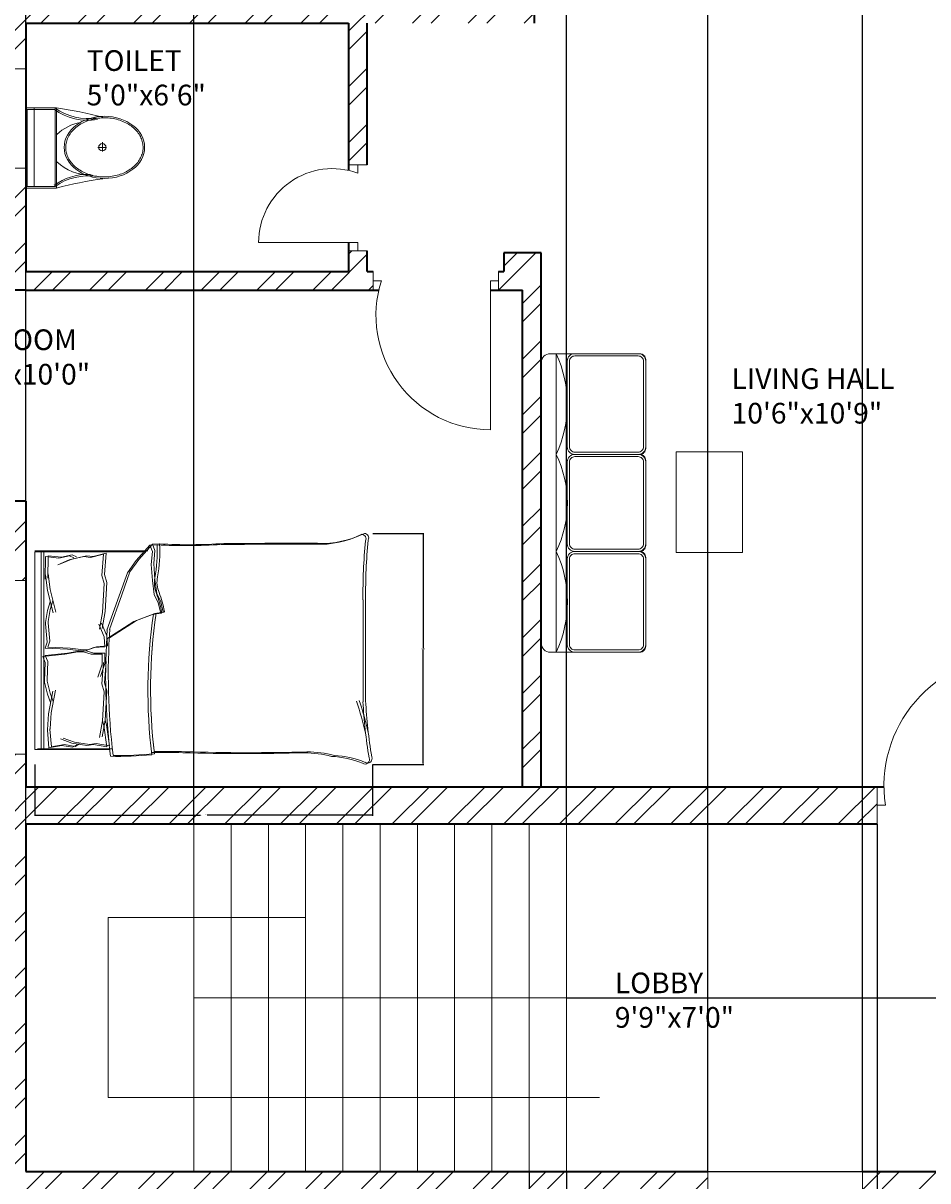
# Model space of a CAD drawing. Units: inches. Extents: x 1513 to 2170, y 1240 to 2288.
# Tile 8 of 10: x 1623 to 1842, y 1801 to 2081. Entities that reach past the tile are written whole.
import ezdxf

# ---------------------------------------------------------------- set-up
doc = ezdxf.new("R2010")
doc.units = ezdxf.units.IN
for name, color, linetype, lineweight in [('A-ANNO-DIMS', 2, 'Continuous', 18), ('A-AREA-IDEN', 7, 'Continuous', 18), ('A-DOOR', 3, 'Continuous', 18), ('A-FLOR-FIXT', 9, 'Continuous', 18), ('A-FLOR-STRS', 7, 'Continuous', 18), ('A-FURN', 8, 'Continuous', 18), ('A-GLAZ', 4, 'Continuous', 18), ('A-WALL', 7, 'Continuous', 35), ('A-WALL-PATT', 252, 'Continuous', 13)]:
    doc.layers.add(name, color=color, linetype=linetype, lineweight=lineweight)
doc.styles.get("Standard").update_dxf_attribs({"font": 'arial.ttf'})
doc.dimstyles.get("Standard").update_dxf_attribs({"dimtxt": 0.18, "dimasz": 0.18, "dimexe": 0.18, "dimexo": 0.0625, "dimgap": 0.09, "dimtad": 0, "dimtih": 1, "dimtoh": 1, "dimdec": 4, "dimzin": 0, "dimdsep": 46, "dimtxsty": 'Standard', "dimcen": 0.09, "dimadec": 0, "dimazin": 0, "dimtfac": 1, "dimtdec": 4, "dimtofl": 0, "dimtmove": 0, "dimatfit": 3, "dimfxl": 1, "dimtolj": 1, "dimtzin": 0, "dimarcsym": 0})

# ---------------------------------------------------------------- blocks, each defined once
blk = doc.blocks.new('A$C31115884')
for p, q in [((283.1, 497.7), (223.4, 497.7)), ((257.5, 466.4), (257.5, 523.2)), ((0, 200), (0, 0)), ((520, 200), (0, 200)), ((10, 190), (10, 10)), ((510, 190), (10, 190)), ((510, 10), (510, 190)), ((520, 0), (520, 200)), ((510, 54.5), (0, 54.5)), ((10, 10), (510, 10)), ((0, 0), (520, 0))]:
    blk.add_line(p, q)
blk.add_circle((255.6, 496.4), 23.6)
for centre, radius, start, end in [((2777.7, -204.6), 2807, 165.4549, 171.71327), ((-294.5, 403.3), 364.7, 324.20913, 9.34987), ((-294.5, 403.3), 374.7, 324.20913, 9.34987), ((805.8, 403.3), 364.7, 170.65013, 215.79087), ((3237, 905), 2807, 188.28673, 194.5451), ((139.5, 406.2), 293.5, 315.84364, 2.65635), ((805.8, 403.3), 374.7, 179.20365, 215.79087), ((383.6, 406.2), 293.5, 190.27735, 224.15636)]:
    blk.add_arc(centre, radius, start, end)
blk.add_ellipse((256.2, 509.9), major_axis=(0, -260.7), ratio=0.772727)
blk.add_open_spline([(256.2, 259.2), (263.1, 259.2), (270, 259.7), (287.8, 262.3), (298.7, 265.1), (319.9, 273.1), (330.2, 278.4), (350.1, 291.1), (359.7, 298.7), (377.7, 315.9), (386.2, 325.5), (401.7, 346.6), (408.8, 358.1), (421.3, 382.5), (426.8, 395.5), (435.9, 422.4), (439.5, 436.4), (444.8, 465.1), (446.5, 479.7), (447.9, 509.2), (447.6, 524), (445, 553.3), (442.7, 567.8), (436.3, 596), (432.1, 609.7), (421.9, 636), (416, 648.6), (402.5, 672.1), (395, 683), (378.6, 703), (369.8, 712.1), (351.1, 728), (341.3, 734.8), (320.9, 746.2), (310.4, 750.7), (288.9, 757.3), (278, 759.4), (256, 761), (245, 760.6), (223.1, 757.2), (212.3, 754.3), (191.1, 746.1), (180.8, 740.7), (160.9, 727.8), (151.4, 720.1), (133.5, 702.7), (125.1, 693), (109.6, 671.7), (102.6, 660.2), (90.2, 635.7), (84.9, 622.7), (76, 595.6), (72.4, 581.6), (67.2, 552.9), (65.6, 538.2), (64.4, 508.8), (64.8, 494), (67.5, 464.7), (69.9, 450.2), (76.6, 422), (80.8, 408.3), (91.1, 382.2), (97.2, 369.7), (110.8, 346.3), (118.4, 335.4), (134.8, 315.6), (143.7, 306.7), (162.4, 290.9), (172.3, 284.2), (192.8, 273), (203.3, 268.6), (224.8, 262.2), (235.8, 260.2), (249.9, 259.3), (253, 259.2), (256.2, 259.2)], degree=3, knots=[0, 0, 0, 0, 0.110105, 0.110105, 0.285049, 0.285049, 0.459994, 0.459994, 0.634938, 0.634938, 0.809882, 0.809882, 0.984827, 0.984827, 1.159771, 1.159771, 1.334715, 1.334715, 1.50966, 1.50966, 1.684604, 1.684604, 1.859549, 1.859549, 2.034493, 2.034493, 2.209437, 2.209437, 2.384382, 2.384382, 2.559326, 2.559326, 2.73427, 2.73427, 2.909215, 2.909215, 3.084159, 3.084159, 3.259103, 3.259103, 3.434048, 3.434048, 3.608992, 3.608992, 3.783936, 3.783936, 3.958881, 3.958881, 4.133825, 4.133825, 4.30877, 4.30877, 4.483714, 4.483714, 4.658658, 4.658658, 4.833603, 4.833603, 5.008547, 5.008547, 5.183491, 5.183491, 5.358436, 5.358436, 5.53338, 5.53338, 5.708324, 5.708324, 5.883269, 5.883269, 6.058213, 6.058213, 6.233158, 6.233158, 6.283185, 6.283185, 6.283185, 6.283185])
blk = doc.blocks.new('BED-DOUBLE')
for p, q in [((30.13, 53.18), (28.38, 53.1, 3.87)), ((30.13, 53.18), (28.38, 53.1, 3.87)), ((0, 51.27), (26.61, 51.27)), ((0, 51.27), (26.61, 51.27)), ((0.64, 51.49), (27.25, 51.49)), ((0.64, 51.49), (27.25, 51.49)), ((1.53, 3.48), (1.53, 51.27)), ((1.53, 3.48), (1.53, 51.27)), ((2.17, 3.7), (2.17, 51.49)), ((2.17, 3.7), (2.17, 51.49)), ((6.4, 49.96), (8.97, 50.56)), ((6.4, 49.96), (8.97, 50.56)), ((8.97, 50.56), (10.02, 50.04)), ((8.97, 50.56), (10.02, 50.04)), ((16.57, 50.7), (13.43, 49.92)), ((16.57, 50.7), (13.43, 49.92)), ((17.21, 50.93), (14.07, 50.15)), ((17.21, 50.93), (14.07, 50.15)), ((16.17, 45.57), (16.57, 50.7)), ((16.17, 45.57), (16.57, 50.7)), ((16.8, 45.8), (17.21, 50.93)), ((16.8, 45.8), (17.21, 50.93)), ((27.74, 52.87), (24.49, 49.16)), ((27.74, 52.87), (24.49, 49.16)), ((28.38, 53.1), (25.13, 49.39)), ((28.38, 53.1), (25.13, 49.39)), ((29.49, 52.95), (27.74, 52.87, 3.87)), ((29.49, 52.95), (27.74, 52.87, 3.87)), ((28.36, 51.33), (27.74, 52.87)), ((28.36, 51.33), (27.74, 52.87)), ((28.05, 48.23), (28.36, 51.33)), ((28.05, 48.23), (28.36, 51.33)), ((29, 51.56), (28.38, 53.1)), ((29, 51.56), (28.38, 53.1)), ((28.69, 48.46), (29, 51.56)), ((28.69, 48.46), (29, 51.56)), ((2.55, 50.11), (2.46, 44.71)), ((2.55, 50.11), (2.46, 44.71)), ((2.55, 50.11), (5.76, 49.73)), ((2.55, 50.11), (5.76, 49.73)), ((3.19, 50.34), (3.1, 44.94)), ((3.19, 50.34), (3.1, 44.94)), ((3.19, 50.34), (6.4, 49.96)), ((3.19, 50.34), (6.4, 49.96)), ((8.25, 49.31), (5.57, 48.13)), ((8.25, 49.31), (5.57, 48.13)), ((5.76, 49.73), (8.33, 50.33)), ((5.76, 49.73), (8.33, 50.33)), ((8.89, 49.54), (6.21, 48.36)), ((8.89, 49.54), (6.21, 48.36)), ((11.83, 50.11), (8.25, 49.31)), ((11.83, 50.11), (8.25, 49.31)), ((8.33, 50.33), (9.38, 49.82)), ((8.33, 50.33), (9.38, 49.82)), ((12.46, 50.34), (8.89, 49.54)), ((12.46, 50.34), (8.89, 49.54)), ((13.43, 49.92), (11.83, 50.11)), ((13.43, 49.92), (11.83, 50.11)), ((14.07, 50.15), (12.46, 50.34)), ((14.07, 50.15), (12.46, 50.34)), ((24.49, 49.16), (22.33, 46.22)), ((24.49, 49.16), (22.33, 46.22)), ((25.13, 49.39), (22.96, 46.45)), ((25.13, 49.39), (22.96, 46.45)), ((28.36, 44.36), (28.05, 48.23)), ((28.36, 44.36), (28.05, 48.23)), ((29, 44.59), (28.69, 48.46)), ((29, 44.59), (28.69, 48.46)), ((2.46, 44.71), (2.54, 45.71)), ((2.46, 44.71), (2.54, 45.71)), ((2.54, 45.71), (3.07, 41.92)), ((2.54, 45.71), (3.07, 41.92)), ((3.1, 44.94), (3.18, 45.94)), ((3.1, 44.94), (3.18, 45.94)), ((3.18, 45.94), (3.71, 42.14)), ((3.18, 45.94), (3.71, 42.14)), ((16.72, 43.61), (16.17, 45.57)), ((16.72, 43.61), (16.17, 45.57)), ((17.36, 43.84), (16.8, 45.8)), ((17.36, 43.84), (16.8, 45.8)), ((22.33, 46.22), (20.31, 40.65)), ((22.33, 46.22), (20.31, 40.65)), ((22.96, 46.45), (20.95, 40.87)), ((22.96, 46.45), (20.95, 40.87)), ((3.71, 42.14), (5.06, 36.72)), ((3.71, 42.14), (5.06, 36.72)), ((16.29, 36.6), (16.72, 43.61)), ((16.29, 36.6), (16.72, 43.61)), ((16.93, 36.83), (17.36, 43.84)), ((16.93, 36.83), (17.36, 43.84)), ((28.83, 40.96), (28.36, 44.36)), ((28.83, 40.95), (28.36, 44.36)), ((29.46, 41.18), (29, 44.59)), ((29.46, 41.18), (29, 44.59)), ((3.07, 41.92), (4.42, 36.5)), ((3.07, 41.92), (4.42, 36.5)), ((3.67, 39.2), (3.07, 37.14)), ((3.67, 39.2), (3.07, 37.14)), ((4.31, 39.43), (3.71, 37.36)), ((4.31, 39.43), (3.71, 37.36)), ((20.31, 40.65), (17.38, 32.31)), ((20.31, 40.65), (17.38, 32.31)), ((20.95, 40.87), (18.02, 32.54)), ((20.95, 40.87), (18.02, 32.54)), ((29.75, 38.94), (28.83, 40.96)), ((29.75, 38.94), (28.83, 40.95)), ((30.39, 39.17), (29.46, 41.18)), ((30.39, 39.17), (29.46, 41.18)), ((31.01, 36.69), (30.39, 39.17)), ((31.01, 36.69), (30.39, 39.17)), ((79.24, 15.06), (79.24, 39.68)), ((79.24, 15.06), (79.24, 39.68)), ((79.88, 15.29), (79.88, 39.91)), ((79.88, 15.29), (79.88, 39.91)), ((3.07, 37.14), (2.53, 34.21)), ((3.07, 37.14), (2.53, 34.21)), ((3.71, 37.36), (3.17, 34.43)), ((3.71, 37.36), (3.17, 34.43)), ((15.62, 32.57), (16.29, 36.6)), ((15.62, 32.57), (16.29, 36.6)), ((16.26, 32.79), (16.93, 36.83)), ((16.26, 32.79), (16.93, 36.83)), ((24.51, 34.68), (29, 36.38)), ((24.51, 34.68), (29, 36.38)), ((28.36, 36.15), (30.37, 36.46)), ((28.36, 36.15), (30.37, 36.46)), ((29, 36.38), (31.01, 36.69)), ((29, 36.38), (31.01, 36.69)), ((30.37, 36.46), (29.75, 38.94)), ((30.37, 36.46), (29.75, 38.94)), ((2.53, 34.21), (2.55, 33.88)), ((2.53, 34.21), (2.55, 33.88)), ((2.55, 33.88), (2.98, 29.46)), ((2.55, 33.88), (2.98, 29.46)), ((3.17, 34.43), (3.19, 34.11)), ((3.17, 34.43), (3.19, 34.11)), ((3.19, 34.11), (3.61, 29.69)), ((3.19, 34.11), (3.61, 29.68)), ((16.74, 30.75), (15.45, 33.82)), ((16.74, 30.75), (15.45, 33.82)), ((17.38, 30.98), (16.09, 34.05)), ((17.38, 30.98), (16.09, 34.05)), ((17.38, 30.26), (23.87, 34.45)), ((17.38, 30.26), (23.87, 34.45)), ((18.02, 30.49), (24.51, 34.68)), ((18.02, 30.49), (24.51, 34.68)), ((23.87, 34.45), (28.36, 36.15)), ((23.87, 34.45), (28.36, 36.15)), ((17.53, 28.53), (17.38, 30.98)), ((17.53, 28.53), (17.38, 30.98)), ((2.98, 29.46), (2.49, 27.98)), ((2.98, 29.46), (2.49, 27.98)), ((2.49, 27.98), (7.86, 27.73)), ((2.49, 27.98), (7.86, 27.73)), ((3.61, 29.69), (3.13, 28.21)), ((3.61, 29.68), (3.13, 28.21)), ((3.13, 28.21), (8.5, 27.96)), ((3.13, 28.21), (8.5, 27.96)), ((12.37, 27.44), (14.21, 28.13)), ((12.37, 27.44), (14.21, 28.13)), ((13.01, 27.67), (14.85, 28.36)), ((13.01, 27.67), (14.85, 28.36)), ((14.21, 28.13), (16.89, 28.3)), ((14.21, 28.13), (16.89, 28.3)), ((14.85, 28.36), (17.53, 28.53)), ((14.85, 28.36), (17.53, 28.53)), ((16.89, 28.3), (16.74, 30.75)), ((16.89, 28.3), (16.74, 30.75)), ((1.87, 25.98), (7.22, 26.56)), ((1.87, 25.98), (7.22, 26.56)), ((2.44, 24.54), (1.87, 25.98)), ((2.44, 24.54), (1.87, 25.98)), ((2.51, 26.21), (7.86, 26.79)), ((2.51, 26.21), (7.86, 26.79)), ((3.08, 24.77), (2.51, 26.21)), ((3.08, 24.77), (2.51, 26.21)), ((7.22, 26.56), (10.4, 27.14)), ((7.22, 26.56), (10.4, 27.14)), ((7.86, 27.73), (11.07, 27.36)), ((7.86, 27.73), (11.07, 27.36)), ((7.86, 26.79), (11.04, 27.37)), ((7.86, 26.79), (11.04, 27.37)), ((8.5, 27.96), (11.71, 27.58)), ((8.5, 27.96), (11.71, 27.58)), ((10.4, 27.14), (11.7, 27.14)), ((10.4, 27.14), (11.7, 27.14)), ((11.04, 27.37), (12.34, 27.37)), ((11.04, 27.37), (12.34, 27.37)), ((11.07, 27.36), (12.37, 27.44)), ((11.07, 27.36), (12.37, 27.44)), ((11.7, 27.14), (13.58, 26.56)), ((11.7, 27.14), (13.58, 26.56)), ((11.71, 27.58), (13.01, 27.67)), ((11.71, 27.58), (13.01, 27.67)), ((12.34, 27.37), (14.22, 26.79)), ((12.34, 27.37), (14.22, 26.79)), ((13.58, 26.56), (16.26, 26.56)), ((13.58, 26.56), (16.26, 26.56)), ((14.22, 26.79), (16.9, 26.79)), ((14.22, 26.79), (16.9, 26.79)), ((16.26, 26.56), (16.26, 24.1)), ((16.26, 26.56), (16.26, 24.1)), ((16.9, 26.79), (16.9, 24.33)), ((16.9, 26.79), (16.9, 24.33)), ((2.3, 20.09), (2.44, 24.54)), ((2.3, 20.09), (2.44, 24.54)), ((2.94, 20.32), (3.08, 24.77)), ((2.94, 20.32), (3.08, 24.77)), ((16.26, 24.1), (15.17, 20.96)), ((16.26, 24.1), (15.17, 20.96)), ((16.9, 24.33), (15.81, 21.19)), ((16.9, 24.33), (15.81, 21.19)), ((16.17, 19.39), (16.57, 24.52)), ((16.17, 19.38), (16.57, 24.52)), ((16.8, 19.61), (17.21, 24.75)), ((16.8, 19.61), (17.21, 24.74)), ((2.3, 19.77), (2.3, 20.09)), ((2.3, 19.77), (2.3, 20.09)), ((3.02, 16.88), (2.3, 19.77)), ((3.02, 16.88), (2.3, 19.77)), ((2.94, 20), (2.94, 20.32)), ((2.94, 20), (2.94, 20.32)), ((3.66, 17.11), (2.94, 20)), ((3.66, 17.11), (2.94, 20)), ((17.36, 17.65), (16.8, 19.61)), ((17.36, 17.65), (16.8, 19.61)), ((3.75, 14.86), (3.02, 16.88)), ((3.75, 14.86), (3.02, 16.88)), ((3.31, 12.11), (4.32, 17.6)), ((3.31, 12.11), (4.32, 17.6)), ((4.39, 15.08), (3.66, 17.11)), ((4.39, 15.08), (3.66, 17.11)), ((3.95, 12.34), (4.96, 17.83)), ((3.95, 12.34), (4.96, 17.83)), ((16.72, 17.42), (16.17, 19.39)), ((16.72, 17.42), (16.17, 19.38)), ((16.29, 10.41), (16.72, 17.42)), ((16.29, 10.41), (16.72, 17.42)), ((16.93, 10.64), (17.36, 17.65)), ((16.93, 10.64), (17.36, 17.65)), ((3.02, 8.29), (3.31, 12.11)), ((3.02, 8.29), (3.31, 12.11)), ((3.66, 8.51), (3.95, 12.34)), ((3.66, 8.51), (3.95, 12.34)), ((3.64, 8.41), (3.66, 8.51)), ((3.64, 8.41), (3.66, 8.51)), ((3.97, 4.13), (3.64, 8.41)), ((3.97, 4.13), (3.64, 8.41)), ((15.62, 6.38), (16.29, 10.41)), ((15.62, 6.38), (16.29, 10.41)), ((16.26, 6.61), (16.93, 10.64)), ((16.26, 6.61), (16.93, 10.64)), ((16.29, 10.41), (16.61, 9.28)), ((16.29, 10.41), (16.61, 9.28)), ((16.61, 9.28), (17.34, 4.18)), ((16.61, 9.28), (17.34, 4.18)), ((16.93, 10.64), (17.25, 9.51)), ((16.93, 10.64), (17.25, 9.51)), ((17.25, 9.51), (17.98, 4.41)), ((17.25, 9.51), (17.98, 4.41)), ((3.01, 8.18), (3.02, 8.29)), ((3.01, 8.18), (3.02, 8.29)), ((3.33, 3.9), (3.01, 8.18)), ((3.33, 3.9), (3.01, 8.18)), ((8.95, 5.05), (6.2, 6.06)), ((8.95, 5.05), (6.2, 6.06)), ((9.59, 5.28), (6.84, 6.29)), ((9.59, 5.28), (6.84, 6.29)), ((18.11, 3.48), (0, 3.48)), ((18.11, 3.48), (0, 3.48)), ((18.75, 3.7), (0.64, 3.7)), ((18.75, 3.7), (0.64, 3.7)), ((3.31, 3.9), (6.49, 4.47)), ((3.31, 3.9), (6.49, 4.47)), ((3.95, 4.12), (7.13, 4.7)), ((3.95, 4.12), (7.13, 4.7)), ((6.49, 4.47), (9.1, 4.04)), ((6.49, 4.47), (9.1, 4.04)), ((7.13, 4.7), (9.74, 4.27)), ((7.13, 4.7), (9.74, 4.27)), ((12.57, 4.47), (8.95, 5.05)), ((12.57, 4.47), (8.95, 5.05)), ((9.1, 4.04), (10.11, 4.62)), ((9.1, 4.04), (10.11, 4.62)), ((13.21, 4.7), (9.59, 5.28)), ((13.21, 4.7), (9.59, 5.28)), ((9.74, 4.27), (10.75, 4.85)), ((9.74, 4.27), (10.75, 4.85)), ((14.16, 4.76), (12.57, 4.47)), ((14.16, 4.76), (12.57, 4.47)), ((14.8, 4.99), (13.21, 4.7)), ((14.8, 4.99), (13.21, 4.7)), ((17.34, 4.18), (14.16, 4.76)), ((17.34, 4.18), (14.16, 4.76)), ((17.98, 4.41), (14.8, 4.99)), ((17.98, 4.41), (14.8, 4.99))]:
    blk.add_line(p, q)
for centre, radius, start, end in [((-6.02, 51.56), 36.18, 349.8763, 2.5657), ((-6.02, 51.56), 36.18, 349.8763, 2.5657), ((36.95, 182.5), 129.5, 266.9791, 273.8365), ((36.95, 182.5), 129.5, 266.9791, 273.8365), ((68.46, -4508.51), 4561.86, 90.00217, 90.28689), ((68.46, -4508.51), 4561.86, 90.00217, 90.28689), ((68.66, 76.16), 23.07, 267.4714, 296.4681), ((68.66, 76.16), 23.07, 267.4714, 296.4681), ((69.3, 76.39), 23.07, 267.4714, 296.4681), ((69.3, 76.39), 23.07, 267.4714, 296.4681), ((78.87, 54.41), 1.1, 332.6588, 86.02), ((78.87, 54.41), 1.1, 332.6588, 86.02), ((212.27, 41.15), 133.04, 174.4998, 180.6351), ((212.27, 41.15), 133.04, 174.4998, 180.6351), ((79.51, 54.64), 1.1, 332.6588, 86.02), ((79.51, 54.64), 1.1, 332.6588, 86.02), ((212.91, 41.38), 133.04, 174.4998, 180.6351), ((212.91, 41.38), 133.04, 174.4998, 180.6351), ((-6.66, 51.33), 36.18, 349.8763, 2.5657), ((-6.66, 51.33), 36.18, 349.8763, 2.5657), ((36.31, 182.27), 129.5, 266.9791, 273.8365), ((36.31, 182.27), 129.5, 266.9791, 273.8365), ((67.82, -4508.74), 4561.86, 90.00217, 90.28689), ((67.82, -4508.74), 4561.86, 90.00217, 90.28689), ((35.06, 43.74), 6.22, 168.6608, 203.7384), ((35.06, 43.74), 6.22, 168.6608, 203.7384), ((35.7, 43.97), 6.22, 168.6608, 203.7384), ((35.7, 43.97), 6.22, 168.6608, 203.7384), ((1.48, 31.15), 29.65, 10.6617, 19.8806), ((1.48, 31.15), 29.65, 10.6617, 19.8806), ((2.12, 31.38), 29.65, 10.6617, 19.8806), ((2.12, 31.38), 29.65, 10.6617, 19.8806), ((156.95, 17.99), 129.02, 171.7845, 186.9006), ((156.95, 17.98), 129.02, 171.7845, 186.9006), ((30.44, 36.64), 0.185, 250.2464, 1.1377), ((30.44, 36.64), 0.185, 250.2464, 1.1377), ((31.08, 36.87), 0.185, 250.2464, 1.1377), ((31.08, 36.87), 0.185, 250.2464, 1.1377), ((156.31, 17.76), 129.02, 171.7845, 186.9006), ((156.31, 17.76), 129.02, 171.7845, 186.9006), ((182.05, 21.36), 164.97, 176.0865, 186.7821), ((182.05, 21.36), 164.97, 176.0865, 186.7821), ((182.69, 21.59), 164.97, 176.0865, 186.7821), ((182.69, 21.59), 164.97, 176.0865, 186.7821), ((-23.72, -17.22), 106.46, 13.3832, 17.7053), ((-23.72, -17.22), 106.46, 13.3832, 17.7053), ((-23.08, -16.99), 106.46, 13.3832, 17.7053), ((-23.08, -16.99), 106.46, 13.3832, 17.7053), ((200.83, 21.43), 121.76, 182.9958, 189.4091), ((200.83, 21.43), 121.76, 182.9958, 189.4091), ((201.47, 21.66), 121.76, 182.9958, 189.4091), ((201.47, 21.66), 121.76, 182.9958, 189.4091), ((31.17, -167.31), 170.11, 88.4762, 91.0082), ((31.17, -167.31), 170.11, 88.4762, 91.0082), ((31.81, -167.08), 170.11, 88.4762, 91.0082), ((31.81, -167.08), 170.11, 88.4762, 91.0082), ((51.25, 485.05), 482.31, 268.2277, 271.7185), ((51.25, 485.05), 482.31, 268.2277, 271.7185), ((65.15, -26.67), 29.63, 76.0648, 88.9113), ((65.15, -26.67), 29.63, 76.0648, 88.9113), ((20.09, 85.16), 83.31, 268.7218, 275.604), ((20.09, 85.16), 83.31, 268.7218, 275.604), ((20.73, 85.39), 83.31, 268.7218, 275.604), ((20.73, 85.39), 83.31, 268.7218, 275.604), ((50.61, 484.82), 482.31, 268.2277, 271.7185), ((50.61, 484.82), 482.31, 268.2277, 271.7185), ((64.51, -26.9), 29.63, 76.0648, 88.9113), ((64.51, -26.9), 29.63, 76.0648, 88.9113), ((70.27, -21.66), 23.56, 67.9751, 86.652), ((70.27, -21.66), 23.56, 67.9751, 86.652), ((70.91, -21.43), 23.56, 67.9751, 86.652), ((70.91, -21.43), 23.56, 67.9751, 86.652), ((79.71, 1.09), 1.09, 236.1736, 23.4781), ((79.71, 1.09), 1.09, 236.1736, 23.4781), ((80.35, 1.32), 1.09, 236.1736, 23.4781), ((80.35, 1.32), 1.09, 236.1736, 23.4781)]:
    blk.add_arc(centre, radius, start, end)
blk = doc.blocks.new('WIN-24')
for p, q in [((0, 24), (9, 24)), ((9, 24), (4.5, 24)), ((4.5, 24), (4.5, 0)), ((4.5, 0), (0, 0)), ((0, 0), (9, 0))]:
    blk.add_line(p, q)
blk = doc.blocks.new('TABLE-COFFEE')
blk.add_lwpolyline([(16.02, 0), (0, 0), (0, 24.35), (16.02, 24.35)], close=True)
blk = doc.blocks.new('*D11')
at = {"layer": 'A-ANNO-DIMS', "color": 0, "lineweight": -2, "transparency": 16777216}
for p, q in [((1626.09, 1901.8), (1626.09, 1889.45)), ((1707.63, 1901.8), (1707.63, 1889.45)), ((1626.27, 1889.63), (1666.04, 1889.63)), ((1707.45, 1889.63), (1667.68, 1889.63))]:
    blk.add_line(p, q, dxfattribs=at)
at = {"layer": 'A-ANNO-DIMS', "color": 0, "transparency": 16777216}
for points in [[(1626.27, 1889.66), (1626.27, 1889.6), (1626.09, 1889.63)], [(1707.45, 1889.66), (1707.45, 1889.6), (1707.63, 1889.63)]]:
    blk.add_solid(points, dxfattribs=at)
at = {"layer": 'Defpoints', "color": 0, "transparency": 16777216}
for p in [(1626.09, 1901.86), (1707.63, 1901.86), (1707.63, 1889.63)]:
    blk.add_point(p, dxfattribs=at)
at = {"layer": 'A-ANNO-DIMS', "color": 0, "transparency": 16777216, "insert": (1666.86, 1889.63), "char_height": 0.18, "attachment_point": 5}
blk.add_mtext('\\A1;BED 82 TYP.', dxfattribs=at)
blk = doc.blocks.new('*D12')
at = {"layer": 'A-ANNO-DIMS', "color": 0, "lineweight": -2, "transparency": 16777216}
for p, q in [((1707.7, 1957.69), (1720.05, 1957.69)), ((1719.87, 1957.51), (1719.87, 1929.96)), ((1719.87, 1902.04), (1719.87, 1929.59)), ((1707.7, 1901.86), (1720.05, 1901.86))]:
    blk.add_line(p, q, dxfattribs=at)
at = {"layer": 'A-ANNO-DIMS', "color": 0, "transparency": 16777216}
for points in [[(1719.84, 1957.51), (1719.9, 1957.51), (1719.87, 1957.69)], [(1719.84, 1902.04), (1719.9, 1902.04), (1719.87, 1901.86)]]:
    blk.add_solid(points, dxfattribs=at)
at = {"layer": 'Defpoints', "color": 0, "transparency": 16777216}
for p in [(1707.63, 1957.69), (1719.87, 1957.69), (1707.63, 1901.86)]:
    blk.add_point(p, dxfattribs=at)
at = {"layer": 'A-ANNO-DIMS', "color": 0, "transparency": 16777216, "insert": (1719.87, 1929.78), "char_height": 0.18, "attachment_point": 5}
blk.add_mtext('\\A1;56 TYP.', dxfattribs=at)
blk = doc.blocks.new('*D25')
at = {"layer": 'A-ANNO-DIMS', "color": 0, "lineweight": -2, "transparency": 16777216}
for p, q in [((1578.87, 2040.54), (1578.87, 2259.81)), ((1579.05, 2259.63), (1810.07, 2259.63)), ((2041.67, 2259.63), (1810.65, 2259.63)), ((2041.85, 2040.54), (2041.85, 2259.81))]:
    blk.add_line(p, q, dxfattribs=at)
at = {"layer": 'A-ANNO-DIMS', "color": 0, "transparency": 16777216}
for points in [[(1579.05, 2259.66), (1579.05, 2259.6), (1578.87, 2259.63)], [(2041.67, 2259.66), (2041.67, 2259.6), (2041.85, 2259.63)]]:
    blk.add_solid(points, dxfattribs=at)
at = {"layer": 'Defpoints', "color": 0, "transparency": 16777216}
for p in [(2041.85, 2259.63), (1578.87, 2040.48), (2041.85, 2040.48)]:
    blk.add_point(p, dxfattribs=at)
at = {"layer": 'A-ANNO-DIMS', "color": 0, "transparency": 16777216, "insert": (1810.36, 2259.63), "char_height": 0.18, "attachment_point": 5}
blk.add_mtext('\\A1;463', dxfattribs=at)
blk = doc.blocks.new('*D32')
at = {"layer": 'A-ANNO-DIMS', "color": 0, "lineweight": -2, "transparency": 16777216}
for p, q in [((1623.87, 1887.54), (1623.87, 2259.81)), ((1624.05, 2259.63), (1643.84, 2259.63)), ((1664.28, 2259.63), (1644.49, 2259.63)), ((1664.46, 1887.54), (1664.46, 2259.81))]:
    blk.add_line(p, q, dxfattribs=at)
at = {"layer": 'A-ANNO-DIMS', "color": 0, "transparency": 16777216}
for points in [[(1624.05, 2259.66), (1624.05, 2259.6), (1623.87, 2259.63)], [(1664.28, 2259.66), (1664.28, 2259.6), (1664.46, 2259.63)]]:
    blk.add_solid(points, dxfattribs=at)
at = {"layer": 'Defpoints', "color": 0, "transparency": 16777216}
for p in [(1664.46, 2259.63), (1623.87, 1887.48), (1664.46, 1887.48)]:
    blk.add_point(p, dxfattribs=at)
at = {"layer": 'A-ANNO-DIMS', "color": 0, "transparency": 16777216, "insert": (1644.16, 2259.63), "char_height": 0.18, "attachment_point": 5}
blk.add_mtext('\\A1;40.6', dxfattribs=at)
blk = doc.blocks.new('*D33')
at = {"layer": 'A-ANNO-DIMS', "color": 0, "lineweight": -2, "transparency": 16777216}
for p, q in [((1664.46, 1887.54), (1664.46, 2259.81)), ((1664.64, 2259.63), (1709.25, 2259.63)), ((1754.28, 2259.63), (1709.68, 2259.63)), ((1754.46, 1887.54), (1754.46, 2259.81))]:
    blk.add_line(p, q, dxfattribs=at)
at = {"layer": 'A-ANNO-DIMS', "color": 0, "transparency": 16777216}
for points in [[(1664.64, 2259.66), (1664.64, 2259.6), (1664.46, 2259.63)], [(1754.28, 2259.66), (1754.28, 2259.6), (1754.46, 2259.63)]]:
    blk.add_solid(points, dxfattribs=at)
at = {"layer": 'Defpoints', "color": 0, "transparency": 16777216}
for p in [(1754.46, 2259.63), (1664.46, 1887.48), (1754.46, 1887.48)]:
    blk.add_point(p, dxfattribs=at)
at = {"layer": 'A-ANNO-DIMS', "color": 0, "transparency": 16777216, "insert": (1709.46, 2259.63), "char_height": 0.18, "attachment_point": 5}
blk.add_mtext('\\A1;90', dxfattribs=at)
blk = doc.blocks.new('*D34')
at = {"layer": 'A-ANNO-DIMS', "color": 0, "lineweight": -2, "transparency": 16777216}
for p, q in [((1745.46, 1803.42), (1745.46, 1344.15)), ((1754.46, 1803.42), (1754.46, 1344.15)), ((1745.64, 1344.33), (1749.81, 1344.33)), ((1754.28, 1344.33), (1750.11, 1344.33))]:
    blk.add_line(p, q, dxfattribs=at)
at = {"layer": 'A-ANNO-DIMS', "color": 0, "transparency": 16777216}
for points in [[(1745.64, 1344.36), (1745.64, 1344.3), (1745.46, 1344.33)], [(1754.28, 1344.36), (1754.28, 1344.3), (1754.46, 1344.33)]]:
    blk.add_solid(points, dxfattribs=at)
at = {"layer": 'Defpoints', "color": 0, "transparency": 16777216}
for p in [(1745.46, 1803.48), (1754.46, 1803.48), (1754.46, 1344.33)]:
    blk.add_point(p, dxfattribs=at)
at = {"layer": 'A-ANNO-DIMS', "color": 0, "transparency": 16777216, "insert": (1749.96, 1344.33), "char_height": 0.18, "attachment_point": 5}
blk.add_mtext('\\A1;9', dxfattribs=at)
blk = doc.blocks.new('*D35')
at = {"layer": 'A-ANNO-DIMS', "color": 0, "lineweight": -2, "transparency": 16777216}
for p, q in [((1754.53, 1845.48), (2087.18, 1845.48)), ((2087, 1845.3), (2087, 1824.66)), ((2087, 1803.66), (2087, 1824.3)), ((1754.53, 1803.48), (2087.18, 1803.48))]:
    blk.add_line(p, q, dxfattribs=at)
at = {"layer": 'A-ANNO-DIMS', "color": 0, "transparency": 16777216}
for points in [[(2086.97, 1845.3), (2087.03, 1845.3), (2087, 1845.48)], [(2086.97, 1803.66), (2087.03, 1803.66), (2087, 1803.48)]]:
    blk.add_solid(points, dxfattribs=at)
at = {"layer": 'Defpoints', "color": 0, "transparency": 16777216}
for p in [(1754.46, 1845.48), (2087, 1845.48), (1754.46, 1803.48)]:
    blk.add_point(p, dxfattribs=at)
at = {"layer": 'A-ANNO-DIMS', "color": 0, "transparency": 16777216, "insert": (2087, 1824.48), "char_height": 0.18, "attachment_point": 5}
blk.add_mtext('\\A1;42', dxfattribs=at)
blk = doc.blocks.new('*D36')
at = {"layer": 'A-ANNO-DIMS', "color": 0, "lineweight": -2, "transparency": 16777216}
for p, q in [((1829.49, 1887.42), (1829.49, 1344.15)), ((1864.51, 1887.42), (1864.51, 1344.15)), ((1829.67, 1344.33), (1846.61, 1344.33)), ((1864.33, 1344.33), (1847.39, 1344.33))]:
    blk.add_line(p, q, dxfattribs=at)
at = {"layer": 'A-ANNO-DIMS', "color": 0, "transparency": 16777216}
for points in [[(1829.67, 1344.36), (1829.67, 1344.3), (1829.49, 1344.33)], [(1864.33, 1344.36), (1864.33, 1344.3), (1864.51, 1344.33)]]:
    blk.add_solid(points, dxfattribs=at)
at = {"layer": 'Defpoints', "color": 0, "transparency": 16777216}
for p in [(1829.49, 1887.48), (1864.51, 1887.48), (1864.51, 1344.33)]:
    blk.add_point(p, dxfattribs=at)
at = {"layer": 'A-ANNO-DIMS', "color": 0, "transparency": 16777216, "insert": (1847, 1344.33), "char_height": 0.18, "attachment_point": 5}
blk.add_mtext('\\A1;35.02', dxfattribs=at)
blk = doc.blocks.new('*D37')
at = {"layer": 'A-ANNO-DIMS', "color": 0, "lineweight": -2, "transparency": 16777216}
for p, q in [((1788.59, 1803.54), (1788.59, 2259.81)), ((1788.77, 2259.63), (1806.89, 2259.63)), ((1825.8, 2259.63), (1807.68, 2259.63)), ((1825.98, 1803.54), (1825.98, 2259.81))]:
    blk.add_line(p, q, dxfattribs=at)
at = {"layer": 'A-ANNO-DIMS', "color": 0, "transparency": 16777216}
for points in [[(1788.77, 2259.66), (1788.77, 2259.6), (1788.59, 2259.63)], [(1825.8, 2259.66), (1825.8, 2259.6), (1825.98, 2259.63)]]:
    blk.add_solid(points, dxfattribs=at)
at = {"layer": 'Defpoints', "color": 0, "transparency": 16777216}
for p in [(1825.98, 2259.63), (1788.59, 1803.48), (1825.98, 1803.48)]:
    blk.add_point(p, dxfattribs=at)
at = {"layer": 'A-ANNO-DIMS', "color": 0, "transparency": 16777216, "insert": (1807.28, 2259.63), "char_height": 0.18, "attachment_point": 5}
blk.add_mtext('\\A1;37.39', dxfattribs=at)

msp = doc.modelspace()

# ---------------------------------------------------------------- hatches: boundary and pattern name
at = {"layer": 'A-WALL-PATT'}
h = msp.add_hatch(dxfattribs=at)
h.set_pattern_fill('ANSI32', color=256)
h.paths.add_polyline_path([(2041.852, 1719.48), (2014.852, 1719.48), (2014.852, 1734.444), (2005.852, 1734.444), (2005.852, 1710.48), (2032.852, 1710.48), (2032.852, 1663.98), (1976.619, 1663.98), (1976.619, 1659.48), (2005.852, 1659.48), (2005.852, 1626.27), (2014.852, 1626.27), (2014.852, 1659.48), (2041.852, 1659.48)])
h.paths.add_polyline_path([(1954.521, 1663.98), (1875.357, 1663.98), (1875.357, 1659.48), (1945.852, 1659.48), (1945.852, 1546.98), (1950.352, 1546.98), (2005.852, 1546.98), (2005.852, 1422.48), (1985.47, 1422.48), (1985.47, 1413.48), (2014.852, 1413.48), (2014.852, 1602.27), (2005.852, 1602.27), (2005.852, 1551.48), (1950.352, 1551.48), (1950.352, 1659.48), (1954.521, 1659.48)])
h.paths.add_polyline_path([(1949.47, 1422.48), (1937.366, 1422.48), (1937.366, 1413.48), (1949.47, 1413.48)], flags=0)
h.paths.add_polyline_path([(1937.366, 1422.48), (1908.866, 1422.48), (1908.866, 1546.98), (1805.486, 1546.98), (1805.486, 1542.48), (1904.366, 1542.48), (1904.366, 1451.2), (1897.222, 1451.2), (1897.222, 1442.2), (1904.366, 1442.2), (1904.366, 1422.48), (1904.366, 1413.48), (1904.366, 1389.48), (1908.866, 1389.48), (1908.866, 1413.48), (1932.866, 1413.48), (1932.866, 1389.48), (1937.366, 1389.48)])
h.paths.add_polyline_path([(1830.254, 1442.2), (1844.144, 1442.2), (1844.144, 1451.2), (1830.254, 1451.2), (1821.254, 1451.2), (1821.254, 1422.48), (1766.366, 1422.48), (1766.366, 1542.48), (1770.265, 1542.48), (1770.265, 1546.98), (1758.774, 1546.98), (1758.774, 1544.73), (1758.774, 1542.48), (1761.866, 1542.48), (1761.866, 1389.48), (1779.454, 1389.48), (1779.454, 1398.48), (1770.866, 1398.48), (1770.866, 1413.48), (1830.254, 1413.48)])
h.paths.add_polyline_path([(1686.156, 1451.2), (1677.156, 1451.2), (1677.156, 1422.48), (1623.866, 1422.48), (1623.866, 1460.073), (1614.866, 1460.073), (1614.866, 1413.48), (1686.156, 1413.48)])
h.paths.add_polyline_path([(1761.866, 1422.48), (1686.156, 1422.48), (1686.156, 1413.48), (1761.866, 1413.48)])
h.paths.add_polyline_path([(1623.866, 1542.48), (1688.266, 1542.48), (1688.266, 1544.73), (1688.266, 1546.98), (1623.866, 1546.98), (1623.866, 1560.442), (1614.866, 1560.442), (1614.866, 1520.073), (1619.366, 1520.073), (1623.866, 1520.073)])
h.paths.add_polyline_path([(1623.866, 1600.98), (1715.366, 1600.98), (1715.366, 1546.98), (1711.055, 1546.98), (1711.055, 1542.48), (1719.866, 1542.48), (1726.867, 1542.48), (1726.867, 1544.73), (1726.867, 1546.98), (1719.866, 1546.98), (1719.866, 1600.98), (1719.866, 1608.301), (1717.616, 1608.301), (1715.366, 1608.301), (1715.366, 1605.48), (1623.866, 1605.48), (1623.866, 1620.254), (1614.866, 1620.254), (1614.866, 1584.442), (1623.866, 1584.442)])
h.paths.add_polyline_path([(1623.866, 1659.48), (1715.366, 1659.48), (1715.366, 1629.2), (1719.866, 1629.2), (1719.866, 1659.48), (1767.866, 1659.48), (1767.866, 1629.2), (1772.366, 1629.2), (1772.366, 1663.98), (1578.866, 1663.98), (1578.866, 1661.73), (1578.866, 1659.48), (1578.866, 1635.48), (1583.366, 1635.48), (1583.366, 1654.98), (1614.866, 1654.98), (1614.866, 1644.254), (1619.366, 1644.254), (1623.866, 1644.254)])
h.paths.add_polyline_path([(1788.587, 1798.98), (1788.587, 1803.48), (1623.866, 1803.48), (1623.866, 1887.48), (1829.49, 1887.48), (1829.49, 1891.98), (1829.49, 1896.48), (1748.366, 1896.48), (1743.866, 1896.48), (1623.866, 1896.48), (1623.866, 1904.333), (1619.366, 1904.333), (1614.866, 1904.333), (1614.866, 1896.48), (1578.866, 1896.48), (1578.866, 1887.48), (1614.866, 1887.48), (1614.866, 1803.48), (1578.866, 1803.48), (1578.866, 1794.48), (1626.866, 1794.48), (1788.587, 1794.48)])
h.paths.add_polyline_path([(1635.866, 1794.48), (1626.866, 1794.48), (1626.866, 1763.627), (1631.366, 1763.627), (1635.866, 1763.627)])
h.paths.add_polyline_path([(1635.866, 1703.627), (1626.866, 1703.627), (1626.866, 1663.98), (1635.866, 1663.98)])
h.paths.add_polyline_path([(1587.866, 2016.48), (1614.866, 2016.48), (1623.866, 2016.48), (1707.767, 2016.48), (1707.767, 2018.73), (1707.767, 2020.98), (1706.366, 2020.98), (1706.366, 2025.944), (1701.866, 2025.944), (1701.866, 2020.98), (1623.866, 2020.98), (1623.866, 2045.903), (1614.866, 2045.903), (1614.866, 2025.48), (1583.366, 2025.48), (1583.366, 2040.48), (1578.866, 2040.48), (1578.866, 2016.48), (1578.866, 1956.48), (1614.866, 1956.48), (1614.866, 1946.333), (1623.866, 1946.333), (1623.866, 1965.48), (1587.866, 1965.48)])
h.paths.add_polyline_path([(1748.366, 2016.48), (1748.366, 2025.48), (1743.866, 2025.48), (1739.366, 2025.48), (1739.366, 2020.98), (1738.09, 2020.98), (1738.09, 2016.48), (1743.866, 2016.48), (1743.866, 1896.48), (1748.366, 1896.48)])
h.paths.add_polyline_path([(1746.736, 2085.48), (1623.866, 2085.48), (1623.866, 2205.48), (1657.136, 2205.48), (1657.136, 2214.48), (1614.866, 2214.48), (1614.866, 2069.903), (1623.866, 2069.903), (1623.866, 2080.98), (1683.866, 2080.98), (1701.866, 2080.98), (1701.866, 2046.743), (1706.366, 2046.743), (1706.366, 2080.98), (1746.736, 2080.98)])
h = msp.add_hatch(dxfattribs=at)
h.set_pattern_fill('ANSI32', color=256)
h.paths.add_polyline_path([(1744.852, 2209.98), (1762.042, 2209.98), (1762.042, 2214.48), (1715.345, 2214.48), (1715.345, 2205.48), (1735.852, 2205.48), (1735.852, 2161.98), (1733.253, 2161.98), (1719.866, 2161.98), (1719.866, 2112.429), (1724.366, 2112.429), (1724.366, 2152.98), (1762.042, 2152.98), (1870.852, 2152.98), (1870.852, 2080.98), (1875.352, 2080.98), (1878.245, 2080.98), (1878.245, 2083.23), (1878.245, 2085.48), (1875.352, 2085.48), (1875.352, 2173.929), (1881.628, 2173.929), (1881.628, 2178.429), (1881.628, 2182.929), (1875.352, 2182.929), (1875.352, 2214.48), (1858.335, 2214.48), (1858.335, 2209.98), (1866.352, 2209.98), (1866.352, 2161.98), (1762.042, 2161.98), (1744.852, 2161.98)])
h.paths.add_polyline_path([(2014.852, 2214.48), (1944.011, 2214.48), (1944.011, 2182.929), (1938.347, 2182.929), (1938.347, 2173.929), (1953.011, 2173.929), (1953.011, 2182.929), (1953.011, 2205.48), (2005.852, 2205.48), (2005.852, 2085.48), (1955.061, 2085.48), (1955.061, 2080.98), (2005.852, 2080.98), (2005.852, 2068.903), (2014.852, 2068.903)])
h.paths.add_polyline_path([(2014.852, 2044.903), (2005.852, 2044.903), (2005.852, 2020.98), (1926.352, 2020.98), (1926.352, 2080.98), (1930.882, 2080.98), (1930.882, 2083.23), (1930.882, 2085.48), (1921.852, 2085.48), (1915.536, 2085.48), (1915.536, 2083.23), (1915.536, 2080.98), (1921.852, 2080.98), (1921.852, 2020.98), (1916.378, 2020.98), (1916.378, 2018.73), (1916.378, 2016.48), (2005.852, 2016.48), (2005.852, 2009.442), (2014.852, 2009.442), (2014.852, 2016.48), (2029.852, 2016.48), (2041.852, 2016.48), (2041.852, 2040.48), (2037.352, 2040.48), (2037.352, 2036.595), (2037.352, 2020.98), (2014.852, 2020.98)])
h.paths.add_polyline_path([(2041.852, 1956.48), (2014.852, 1956.48), (2014.852, 1963.797), (2005.852, 1963.797), (2005.852, 1947.48), (2032.852, 1947.48), (2032.852, 1896.48), (1978.852, 1896.48), (1978.852, 1891.98), (1978.852, 1887.48), (2005.852, 1887.48), (2005.852, 1862.401), (2014.852, 1862.401), (2014.852, 1887.48), (2037.352, 1887.48), (2037.352, 1863.48), (2041.852, 1863.48), (2041.852, 1887.48), (2041.852, 1896.48)], flags=17)
h.paths.add_polyline_path([(1885.852, 1896.48), (1885.852, 1920.48), (1878.866, 1920.48), (1878.866, 2016.48), (1881.925, 2016.48), (1881.925, 2018.73), (1881.925, 2020.98), (1874.366, 2020.98), (1874.366, 1896.48), (1864.508, 1896.48), (1864.508, 1887.48), (1876.852, 1887.48), (1876.852, 1855.773), (1885.852, 1855.773), (1885.852, 1868.947), (1942.852, 1868.947), (1942.852, 1803.48), (1885.852, 1803.48), (1885.852, 1817.861), (1876.852, 1817.861), (1876.852, 1803.48), (1825.976, 1803.48), (1825.976, 1798.98), (1825.976, 1794.48), (1832.366, 1794.48), (1832.366, 1663.98), (1832.366, 1659.48), (1841.939, 1659.48), (1841.939, 1661.73), (1841.939, 1663.98), (1836.866, 1663.98), (1836.866, 1794.48), (1992.866, 1794.48), (2005.852, 1794.48), (2005.852, 1784.304), (2010.352, 1784.304), (2014.852, 1784.304), (2014.852, 1794.48), (2041.852, 1794.48), (2041.852, 1803.48), (2014.852, 1803.48), (2014.852, 1838.401), (2005.852, 1838.401), (2005.852, 1803.48), (1951.852, 1803.48), (1951.852, 1887.48), (1956.114, 1887.48), (1956.114, 1891.98), (1956.114, 1896.48), (1951.852, 1896.48), (1951.852, 1920.48), (1947.352, 1920.48), (1947.352, 1896.48), (1942.852, 1896.48), (1942.852, 1877.947), (1885.852, 1877.947)])

# ---------------------------------------------------------------- linework, layer by layer
at = {"layer": 'A-DOOR'}
for p, q in [((1701.866, 2046.743), (1706.366, 2046.743)), ((1706.366, 2046.743), (1704.116, 2046.743)), ((1704.116, 2046.743), (1704.116, 2044.743)), ((1704.116, 2027.944), (1680.116, 2027.944)), ((1706.366, 2025.944), (1701.866, 2025.944)), ((1701.866, 2025.944), (1704.116, 2025.944)), ((1704.116, 2025.944), (1704.116, 2027.944)), ((1707.767, 2020.98), (1707.767, 2016.48)), ((1738.09, 2020.98), (1738.09, 2016.48)), ((1707.767, 2016.48), (1707.767, 2018.73)), ((1707.767, 2018.73), (1709.767, 2018.73)), ((1738.09, 2018.73), (1736.09, 2018.73)), ((1736.09, 2018.73), (1736.09, 1982.73)), ((1738.09, 2016.48), (1738.09, 2018.73)), ((1829.49, 1896.48), (1829.49, 1887.48)), ((1829.49, 1887.48), (1829.49, 1891.98)), ((1829.49, 1891.98), (1831.49, 1891.98)), ((1788.587, 1803.48), (1788.587, 1794.48)), ((1825.976, 1794.48), (1825.976, 1803.48)), ((1825.976, 1803.48), (1825.976, 1798.98))]:
    msp.add_line(p, q, dxfattribs=at)
for centre, radius, start, end in [((1697.995, 2027.944), 17.879, 69.98017, 180), ((1736.09, 2010.353), 27.624, 162.34889, 270), ((1862.508, 1896.616), 31.363, 90, 188.50132)]:
    msp.add_arc(centre, radius, start, end, dxfattribs=at)
at = {"layer": 'A-FLOR-STRS'}
for p, q in [((1664.464, 1803.48), (1664.464, 1887.48)), ((1673.464, 1803.48), (1673.464, 1887.48)), ((1682.464, 1803.48), (1682.464, 1887.48)), ((1691.464, 1803.48), (1691.464, 1887.48)), ((1700.464, 1803.48), (1700.464, 1887.48)), ((1709.464, 1803.48), (1709.464, 1887.48)), ((1718.464, 1803.48), (1718.464, 1887.48)), ((1727.464, 1803.48), (1727.464, 1887.48)), ((1736.464, 1803.48), (1736.464, 1887.48)), ((1745.464, 1803.48), (1745.464, 1887.48)), ((1754.464, 1803.48), (1754.464, 1887.48)), ((1643.794, 1821.352), (1643.794, 1864.849)), ((1643.794, 1864.849), (1691.464, 1864.849)), ((1664.464, 1845.48), (1754.464, 1845.48)), ((1762.473, 1821.352), (1643.794, 1821.352))]:
    msp.add_line(p, q, dxfattribs=at)
at = {"layer": 'A-FURN'}
for p, q in [((1626.086, 1953.445), (1626.726, 1953.445)), ((1626.086, 1953.216), (1626.086, 1905.426))]:
    msp.add_line(p, q, dxfattribs=at)
at = {"layer": 'A-FURN', "ltscale": 0.03}
msp.add_lwpolyline([(1773.612, 1978.227), (1773.612, 1999.669, 0.4142136), (1772.169, 2001.111), (1750.53, 2001.111, 0.4142136), (1748.366, 1998.947), (1748.366, 1931.142, 0.4142136), (1750.53, 1928.978), (1772.169, 1928.978, 0.4142136), (1773.612, 1930.421), (1773.612, 1951.863, 0.4142136), (1772.169, 1953.306, -1), (1772.169, 1953.341, 0.4142136), (1773.612, 1954.784), (1773.612, 1975.306, 0.4142136), (1772.169, 1976.749, -1), (1772.169, 1976.784, 0.4142136)], format="xyb", close=True, dxfattribs=at)
at = {"layer": 'A-FURN'}
msp.add_lwpolyline([(1751.972, 2001.111), (1751.972, 1928.978)], dxfattribs=at)
for points in [[(1771.809, 2001.111), (1756.481, 2001.111, 0.4142136), (1754.677, 1999.308), (1754.677, 1978.57, 0.4142136), (1756.481, 1976.766), (1771.809, 1976.766, 0.4142136), (1773.612, 1978.57), (1773.612, 1999.308, 0.4142136)], [(1771.809, 2000.57), (1756.481, 2000.57, 0.4142136), (1755.218, 1999.308), (1755.218, 1978.57, 0.4142136), (1756.481, 1977.307), (1771.809, 1977.307, 0.4142136), (1773.071, 1978.57), (1773.071, 1999.308, 0.4142136)], [(1771.809, 1953.323), (1756.481, 1953.323, -0.4142136), (1754.677, 1955.127), (1754.677, 1974.963, -0.4142136), (1756.481, 1976.766), (1771.809, 1976.766, -0.4142136), (1773.612, 1974.963), (1773.612, 1955.127, -0.4142136)], [(1771.809, 1953.864), (1756.481, 1953.864, -0.4142136), (1755.218, 1955.127), (1755.218, 1974.963, -0.4142136), (1756.481, 1976.226), (1771.809, 1976.226, -0.4142136), (1773.071, 1974.963), (1773.071, 1955.127, -0.4142136)], [(1771.809, 1953.323), (1756.481, 1953.323, 0.4142136), (1754.677, 1951.52), (1754.677, 1930.782, 0.4142136), (1756.481, 1928.978), (1771.809, 1928.978, 0.4142136), (1773.612, 1930.782), (1773.612, 1951.52, 0.4142136)], [(1771.809, 1952.782), (1756.481, 1952.782, 0.4142136), (1755.218, 1951.52), (1755.218, 1930.782, 0.4142136), (1756.481, 1929.519), (1771.809, 1929.519, 0.4142136), (1773.071, 1930.782), (1773.071, 1951.52, 0.4142136)]]:
    msp.add_lwpolyline(points, format="xyb", close=True, dxfattribs=at)
for centre, radius, start, end in [((1725.974, 1988.939), 28.706, 334.91063, 25.08937), ((1728.078, 1965.045), 26.614, 333.869, 26.131), ((1726.275, 1941.151), 28.434, 334.65382, 25.34618)]:
    msp.add_arc(centre, radius, start, end, dxfattribs=at)
at = {"layer": 'A-GLAZ'}
for p, q in [((1614.866, 1946.333), (1623.866, 1946.333)), ((1614.866, 1904.333), (1623.866, 1904.333)), ((1623.866, 1904.333), (1619.366, 1904.333))]:
    msp.add_line(p, q, dxfattribs=at)
at = {"layer": 'A-WALL'}
for p, q in [((1746.736, 2080.98), (1746.736, 2085.48)), ((1623.866, 2080.98), (1701.866, 2080.98)), ((1623.866, 2080.98), (1623.866, 2020.98)), ((1623.866, 2080.98), (1683.866, 2080.98)), ((1683.866, 2080.98), (1701.866, 2080.98)), ((1701.866, 2080.98), (1701.866, 2045.399)), ((1706.366, 2046.743), (1706.366, 2080.98)), ((1701.866, 2027.944), (1701.866, 2020.98)), ((1706.366, 2020.98), (1706.366, 2025.944)), ((1743.866, 2025.48), (1739.366, 2025.48)), ((1739.366, 2025.48), (1739.366, 2020.98)), ((1748.366, 2025.48), (1743.866, 2025.48)), ((1748.366, 2016.48), (1748.366, 2025.48)), ((1623.866, 2020.98), (1701.866, 2020.98)), ((1706.366, 2020.98), (1707.767, 2020.98)), ((1738.09, 2020.98), (1739.366, 2020.98)), ((1623.866, 2016.48), (1614.866, 2016.48)), ((1623.866, 2016.48), (1709.154, 2016.48)), ((1701.866, 2016.48), (1706.366, 2016.48)), ((1736.09, 2016.48), (1743.866, 2016.48)), ((1743.866, 1896.48), (1743.866, 2016.48)), ((1748.366, 1896.48), (1748.366, 2016.48)), ((1623.866, 1965.48), (1587.866, 1965.48)), ((1623.866, 1965.48), (1623.866, 1896.48)), ((1623.866, 1896.48), (1831.145, 1896.48)), ((1623.866, 1896.48), (1743.866, 1896.48)), ((1743.866, 1896.48), (1748.366, 1896.48)), ((1748.366, 1896.48), (1831.145, 1896.48)), ((1623.866, 1887.48), (1623.866, 1803.48)), ((1623.866, 1887.48), (1829.49, 1887.48)), ((1623.866, 1803.48), (1788.587, 1803.48)), ((1825.976, 1803.48), (1876.852, 1803.48))]:
    msp.add_line(p, q, dxfattribs=at)

# ---------------------------------------------------------------- block references
at = {"layer": 'A-FLOR-FIXT', "xscale": 0.0372717239612423, "yscale": 0.0372717239612423, "zscale": 0.0372717239612423, "rotation": 270}
msp.add_blockref('A$C31115884', (1623.866, 2060.516), dxfattribs=at)
at = {"layer": 'A-FURN'}
for name, p in [('TABLE-COFFEE', (1780.99, 1953.08)), ('BED-DOUBLE', (1626.09, 1901.95))]:
    msp.add_blockref(name, p, dxfattribs=at)
at = {"layer": 'A-GLAZ'}
msp.add_blockref('WIN-24', (1614.863, 2045.903), dxfattribs=at)

# ---------------------------------------------------------------- texts
at = {"layer": 'A-AREA-IDEN', "char_height": 5, "attachment_point": 1}
for s, width, insert in [('TOILET\\P5\'0"x6\'6"', 119.81939, (1638.582, 2074.441)), ('BEDROOM\\P10\'0"x10\'0"', 185.75698, (1603.048, 2006.976)), ('LIVING HALL\\P10\'6"x10\'9"', 257.24596, (1794.359, 1997.563)), ('LOBBY\\P9\'9"x7\'0"', 176.7034, (1766.149, 1851.561))]:
    msp.add_mtext_dynamic_manual_height_columns(s, width=width, gutter_width=12.5, heights=[0], dxfattribs=dict(at, insert=insert))

# ---------------------------------------------------------------- dimensions: what is measured, and where the dimension line sits
at = {"layer": 'A-ANNO-DIMS'}
for base, p1, p2, override, picture, middle in [((2041.852, 2259.63), (1578.866, 2040.48), (2041.852, 2040.48), {"dimdec": 0, "dimlfac": 1, "dimrnd": 0, "dimzin": 0, "dimdsep": 46, "dimlunit": 2}, '*D25', (1810.359, 2259.63)), ((1664.464, 2259.63), (1623.866, 1887.48), (1664.464, 1887.48), {"dimdec": 1, "dimlfac": 1, "dimrnd": 0, "dimzin": 0, "dimdsep": 46, "dimlunit": 2}, '*D32', (1644.165, 2259.63)), ((1754.464, 2259.63), (1664.464, 1887.48), (1754.464, 1887.48), {"dimdec": 0, "dimlfac": 1, "dimrnd": 0, "dimzin": 0, "dimdsep": 46, "dimlunit": 2}, '*D33', (1709.464, 2259.63)), ((1825.976, 2259.63), (1788.587, 1803.48), (1825.976, 1803.48), {"dimdec": 2, "dimlfac": 1, "dimrnd": 0, "dimzin": 0, "dimdsep": 46, "dimlunit": 2}, '*D37', (1807.281, 2259.63)), ((1864.508, 1344.33), (1829.49, 1887.48), (1864.508, 1887.48), {"dimdec": 2, "dimlfac": 1, "dimrnd": 0, "dimzin": 0, "dimdsep": 46, "dimlunit": 2}, '*D36', (1846.999, 1344.33)), ((1754.464, 1344.33), (1745.464, 1803.48), (1754.464, 1803.48), {"dimdec": 0, "dimlfac": 1, "dimrnd": 0, "dimzin": 0, "dimdsep": 46, "dimlunit": 2}, '*D34', (1749.964, 1344.33))]:
    dim = msp.add_linear_dim(base=base, p1=p1, p2=p2, dimstyle='Standard', override=override, dxfattribs=at)
    dim.commit()
    dim.dimension.update_dxf_attribs({"geometry": picture, "text_midpoint": middle})
dim = msp.add_linear_dim(base=(1719.867, 1957.689), p1=(1707.635, 1901.865), p2=(1707.635, 1957.689), angle=90, text='<> TYP.', dimstyle='Standard', override={"dimdec": 0, "dimlfac": 1, "dimrnd": 0, "dimzin": 0, "dimdsep": 46, "dimlunit": 2}, dxfattribs=at)
dim.commit()
dim.dimension.update_dxf_attribs({"geometry": '*D12', "text_midpoint": (1719.867, 1929.777)})
dim = msp.add_linear_dim(base=(1707.635, 1889.632), p1=(1626.086, 1901.865), p2=(1707.635, 1901.865), text='BED <> TYP.', dimstyle='Standard', override={"dimdec": 0, "dimlfac": 1, "dimrnd": 0, "dimzin": 0, "dimdsep": 46, "dimlunit": 2}, dxfattribs=at)
dim.commit()
dim.dimension.update_dxf_attribs({"geometry": '*D11', "text_midpoint": (1666.861, 1889.632)})
dim = msp.add_linear_dim(base=(2087.002, 1845.48), p1=(1754.464, 1803.48), p2=(1754.464, 1845.48), angle=90, dimstyle='Standard', override={"dimdec": 0, "dimlfac": 1, "dimrnd": 0, "dimzin": 0, "dimdsep": 46, "dimlunit": 2}, dxfattribs=at)
dim.commit()
dim.dimension.update_dxf_attribs({"geometry": '*D35', "text_midpoint": (2087.002, 1824.48)})

doc.saveas('drawing.dxf')
